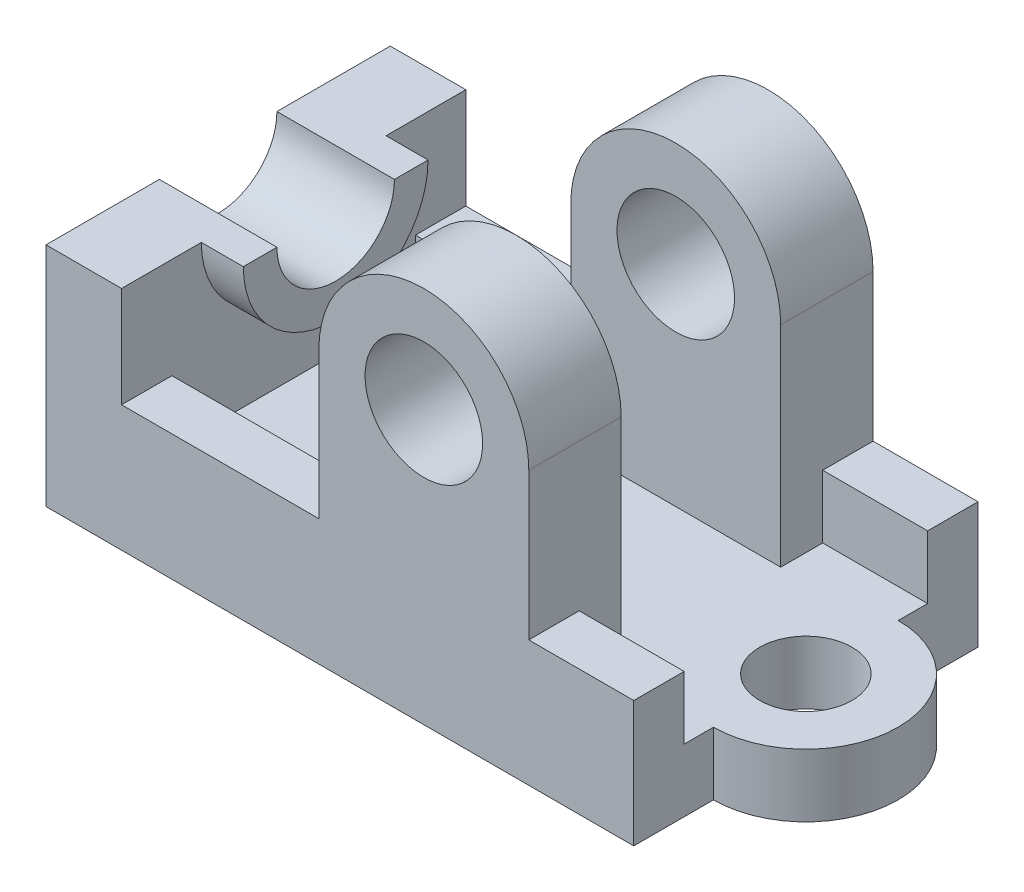
ISO-10303-21;
HEADER;
FILE_DESCRIPTION(('STEP AP214'),'2;1');
FILE_NAME('part.step','',(''),(''),'','','');
FILE_SCHEMA(('AUTOMOTIVE_DESIGN { 1 0 10303 214 1 1 1 1 }'));
ENDSEC;
DATA;
#1=APPLICATION_CONTEXT('core data for automotive mechanical design processes');
#2=APPLICATION_PROTOCOL_DEFINITION('international standard','automotive_design',2000,#1);
#3=PRODUCT_CONTEXT('',#1,'mechanical');
#4=PRODUCT('Part','Part','',(#3));
#5=PRODUCT_RELATED_PRODUCT_CATEGORY('part','',(#4));
#6=PRODUCT_DEFINITION_FORMATION('','',#4);
#7=PRODUCT_DEFINITION_CONTEXT('part definition',#1,'design');
#8=PRODUCT_DEFINITION('design','',#6,#7);
#9=PRODUCT_DEFINITION_SHAPE('','',#8);
#10=(LENGTH_UNIT() NAMED_UNIT(*) SI_UNIT(.MILLI.,.METRE.));
#11=(NAMED_UNIT(*) PLANE_ANGLE_UNIT() SI_UNIT($,.RADIAN.));
#12=(NAMED_UNIT(*) SI_UNIT($,.STERADIAN.) SOLID_ANGLE_UNIT());
#13=UNCERTAINTY_MEASURE_WITH_UNIT(LENGTH_MEASURE(1.E-05),#10,'distance_accuracy_value','');
#14=(GEOMETRIC_REPRESENTATION_CONTEXT(3) GLOBAL_UNCERTAINTY_ASSIGNED_CONTEXT((#13)) GLOBAL_UNIT_ASSIGNED_CONTEXT((#10,
#11,#12)) REPRESENTATION_CONTEXT('',''));
#15=CARTESIAN_POINT('',(0.,0.,0.));
#16=DIRECTION('',(0.,0.,1.));
#17=DIRECTION('',(1.,0.,0.));
#18=AXIS2_PLACEMENT_3D('',#15,#16,#17);
#19=CARTESIAN_POINT('',(140.,30.,41.));
#20=DIRECTION('',(-1.,0.,0.));
#21=DIRECTION('',(0.,0.,1.));
#22=AXIS2_PLACEMENT_3D('',#19,#20,#21);
#23=PLANE('',#22);
#24=DIRECTION('',(0.,0.,-1.));
#25=VECTOR('',#24,1.);
#26=CARTESIAN_POINT('',(140.,15.,41.));
#27=LINE('',#26,#25);
#28=CARTESIAN_POINT('',(140.,15.,-22.));
#29=VERTEX_POINT('',#28);
#30=CARTESIAN_POINT('',(140.,15.,-29.));
#31=VERTEX_POINT('',#30);
#32=EDGE_CURVE('E247',#29,#31,#27,.T.);
#33=ORIENTED_EDGE('',*,*,#32,.F.);
#34=DIRECTION('',(0.,-1.,0.));
#35=VECTOR('',#34,1.);
#36=CARTESIAN_POINT('',(140.,15.,-22.));
#37=LINE('',#36,#35);
#38=CARTESIAN_POINT('',(140.,0.,-22.));
#39=VERTEX_POINT('',#38);
#40=EDGE_CURVE('E229',#29,#39,#37,.T.);
#41=ORIENTED_EDGE('',*,*,#40,.T.);
#42=DIRECTION('',(0.,0.,-1.));
#43=VECTOR('',#42,1.);
#44=CARTESIAN_POINT('',(140.,0.,41.));
#45=LINE('',#44,#43);
#46=CARTESIAN_POINT('',(140.,0.,-41.));
#47=VERTEX_POINT('',#46);
#48=EDGE_CURVE('E293',#39,#47,#45,.T.);
#49=ORIENTED_EDGE('',*,*,#48,.T.);
#50=DIRECTION('',(0.,1.,0.));
#51=VECTOR('',#50,1.);
#52=CARTESIAN_POINT('',(140.,30.,-41.));
#53=LINE('',#52,#51);
#54=CARTESIAN_POINT('',(140.,30.,-41.));
#55=VERTEX_POINT('',#54);
#56=EDGE_CURVE('E272',#47,#55,#53,.T.);
#57=ORIENTED_EDGE('',*,*,#56,.T.);
#58=DIRECTION('',(0.,0.,-1.));
#59=VECTOR('',#58,1.);
#60=CARTESIAN_POINT('',(140.,30.,-29.));
#61=LINE('',#60,#59);
#62=CARTESIAN_POINT('',(140.,30.,-29.));
#63=VERTEX_POINT('',#62);
#64=EDGE_CURVE('E331',#63,#55,#61,.T.);
#65=ORIENTED_EDGE('',*,*,#64,.F.);
#66=DIRECTION('',(0.,-1.,0.));
#67=VECTOR('',#66,1.);
#68=CARTESIAN_POINT('',(140.,15.,-29.));
#69=LINE('',#68,#67);
#70=EDGE_CURVE('E325',#63,#31,#69,.T.);
#71=ORIENTED_EDGE('',*,*,#70,.T.);
#72=EDGE_LOOP('',(#33,#41,#49,#57,#65,#71));
#73=FACE_BOUND('',#72,.T.);
#74=ADVANCED_FACE('F41',(#73),#23,.F.);
#75=CARTESIAN_POINT('',(0.,54.,41.));
#76=DIRECTION('',(0.,-1.,0.));
#77=DIRECTION('',(0.,0.,-1.));
#78=AXIS2_PLACEMENT_3D('',#75,#76,#77);
#79=PLANE('',#78);
#80=DIRECTION('',(0.,0.,-1.));
#81=VECTOR('',#80,1.);
#82=CARTESIAN_POINT('',(0.,54.,41.));
#83=LINE('',#82,#81);
#84=CARTESIAN_POINT('',(0.,54.,-14.));
#85=VERTEX_POINT('',#84);
#86=CARTESIAN_POINT('',(0.,54.,-41.));
#87=VERTEX_POINT('',#86);
#88=EDGE_CURVE('E283',#85,#87,#83,.T.);
#89=ORIENTED_EDGE('',*,*,#88,.F.);
#90=DIRECTION('',(1.,0.,0.));
#91=VECTOR('',#90,1.);
#92=CARTESIAN_POINT('',(18.,54.,-14.));
#93=LINE('',#92,#91);
#94=CARTESIAN_POINT('',(28.,54.,-14.));
#95=VERTEX_POINT('',#94);
#96=EDGE_CURVE('E61',#85,#95,#93,.T.);
#97=ORIENTED_EDGE('',*,*,#96,.T.);
#98=DIRECTION('',(0.,0.,-1.));
#99=VECTOR('',#98,1.);
#100=CARTESIAN_POINT('',(28.,54.,0.));
#101=LINE('',#100,#99);
#102=CARTESIAN_POINT('',(28.,54.,-22.));
#103=VERTEX_POINT('',#102);
#104=EDGE_CURVE('E537',#95,#103,#101,.T.);
#105=ORIENTED_EDGE('',*,*,#104,.T.);
#106=DIRECTION('',(1.,0.,0.));
#107=VECTOR('',#106,1.);
#108=CARTESIAN_POINT('',(18.,54.,-22.));
#109=LINE('',#108,#107);
#110=CARTESIAN_POINT('',(18.,54.,-22.));
#111=VERTEX_POINT('',#110);
#112=EDGE_CURVE('E490',#111,#103,#109,.T.);
#113=ORIENTED_EDGE('',*,*,#112,.F.);
#114=DIRECTION('',(0.,0.,-1.));
#115=VECTOR('',#114,1.);
#116=CARTESIAN_POINT('',(18.,54.,41.));
#117=LINE('',#116,#115);
#118=CARTESIAN_POINT('',(18.,54.,-41.));
#119=VERTEX_POINT('',#118);
#120=EDGE_CURVE('E289',#111,#119,#117,.T.);
#121=ORIENTED_EDGE('',*,*,#120,.T.);
#122=DIRECTION('',(-1.,0.,0.));
#123=VECTOR('',#122,1.);
#124=CARTESIAN_POINT('',(0.,54.,-41.));
#125=LINE('',#124,#123);
#126=EDGE_CURVE('E280',#119,#87,#125,.T.);
#127=ORIENTED_EDGE('',*,*,#126,.T.);
#128=EDGE_LOOP('',(#89,#97,#105,#113,#121,#127));
#129=FACE_BOUND('',#128,.T.);
#130=ADVANCED_FACE('F446',(#129),#79,.F.);
#131=CARTESIAN_POINT('',(140.,30.,-29.));
#132=DIRECTION('',(0.,1.,0.));
#133=DIRECTION('',(0.,0.,1.));
#134=AXIS2_PLACEMENT_3D('',#131,#132,#133);
#135=PLANE('',#134);
#136=DIRECTION('',(0.,0.,1.));
#137=VECTOR('',#136,1.);
#138=CARTESIAN_POINT('',(65.,30.,-29.));
#139=LINE('',#138,#137);
#140=CARTESIAN_POINT('',(65.,30.,-41.));
#141=VERTEX_POINT('',#140);
#142=CARTESIAN_POINT('',(65.,30.,-29.));
#143=VERTEX_POINT('',#142);
#144=EDGE_CURVE('E406',#141,#143,#139,.T.);
#145=ORIENTED_EDGE('',*,*,#144,.F.);
#146=DIRECTION('',(1.,0.,0.));
#147=VECTOR('',#146,1.);
#148=CARTESIAN_POINT('',(140.,30.,-41.));
#149=LINE('',#148,#147);
#150=CARTESIAN_POINT('',(18.,30.,-41.));
#151=VERTEX_POINT('',#150);
#152=EDGE_CURVE('E329',#151,#141,#149,.T.);
#153=ORIENTED_EDGE('',*,*,#152,.F.);
#154=DIRECTION('',(0.,0.,-1.));
#155=VECTOR('',#154,1.);
#156=CARTESIAN_POINT('',(18.,30.,-29.));
#157=LINE('',#156,#155);
#158=CARTESIAN_POINT('',(18.,30.,-29.));
#159=VERTEX_POINT('',#158);
#160=EDGE_CURVE('E327',#159,#151,#157,.T.);
#161=ORIENTED_EDGE('',*,*,#160,.F.);
#162=DIRECTION('',(1.,0.,0.));
#163=VECTOR('',#162,1.);
#164=CARTESIAN_POINT('',(140.,30.,-29.));
#165=LINE('',#164,#163);
#166=EDGE_CURVE('E326',#159,#143,#165,.T.);
#167=ORIENTED_EDGE('',*,*,#166,.T.);
#168=EDGE_LOOP('',(#145,#153,#161,#167));
#169=FACE_BOUND('',#168,.T.);
#170=ADVANCED_FACE('F453',(#169),#135,.T.);
#171=CARTESIAN_POINT('',(0.,0.,-29.));
#172=DIRECTION('',(0.,0.,1.));
#173=DIRECTION('',(1.,0.,0.));
#174=AXIS2_PLACEMENT_3D('',#171,#172,#173);
#175=PLANE('',#174);
#176=DIRECTION('',(0.,-1.,0.));
#177=VECTOR('',#176,1.);
#178=CARTESIAN_POINT('',(65.,0.,-29.));
#179=LINE('',#178,#177);
#180=CARTESIAN_POINT('',(65.,15.,-29.));
#181=VERTEX_POINT('',#180);
#182=EDGE_CURVE('E11',#143,#181,#179,.T.);
#183=ORIENTED_EDGE('',*,*,#182,.F.);
#184=ORIENTED_EDGE('',*,*,#166,.F.);
#185=DIRECTION('',(0.,1.,0.));
#186=VECTOR('',#185,1.);
#187=CARTESIAN_POINT('',(18.,15.,-29.));
#188=LINE('',#187,#186);
#189=CARTESIAN_POINT('',(18.,15.,-29.));
#190=VERTEX_POINT('',#189);
#191=EDGE_CURVE('E320',#190,#159,#188,.T.);
#192=ORIENTED_EDGE('',*,*,#191,.F.);
#193=DIRECTION('',(-1.,0.,0.));
#194=VECTOR('',#193,1.);
#195=CARTESIAN_POINT('',(140.,15.,-29.));
#196=LINE('',#195,#194);
#197=EDGE_CURVE('E319',#181,#190,#196,.T.);
#198=ORIENTED_EDGE('',*,*,#197,.F.);
#199=EDGE_LOOP('',(#183,#184,#192,#198));
#200=FACE_BOUND('',#199,.T.);
#201=ADVANCED_FACE('F604',(#200),#175,.T.);
#202=CARTESIAN_POINT('',(18.,30.,29.));
#203=DIRECTION('',(0.,1.,0.));
#204=DIRECTION('',(0.,0.,1.));
#205=AXIS2_PLACEMENT_3D('',#202,#203,#204);
#206=PLANE('',#205);
#207=DIRECTION('',(0.,0.,1.));
#208=VECTOR('',#207,1.);
#209=CARTESIAN_POINT('',(65.,30.,29.));
#210=LINE('',#209,#208);
#211=CARTESIAN_POINT('',(65.,30.,29.));
#212=VERTEX_POINT('',#211);
#213=CARTESIAN_POINT('',(65.,30.,41.));
#214=VERTEX_POINT('',#213);
#215=EDGE_CURVE('E392',#212,#214,#210,.T.);
#216=ORIENTED_EDGE('',*,*,#215,.F.);
#217=DIRECTION('',(-1.,0.,0.));
#218=VECTOR('',#217,1.);
#219=CARTESIAN_POINT('',(18.,30.,29.));
#220=LINE('',#219,#218);
#221=CARTESIAN_POINT('',(18.,30.,29.));
#222=VERTEX_POINT('',#221);
#223=EDGE_CURVE('E348',#212,#222,#220,.T.);
#224=ORIENTED_EDGE('',*,*,#223,.T.);
#225=DIRECTION('',(0.,0.,1.));
#226=VECTOR('',#225,1.);
#227=CARTESIAN_POINT('',(18.,30.,29.));
#228=LINE('',#227,#226);
#229=CARTESIAN_POINT('',(18.,30.,41.));
#230=VERTEX_POINT('',#229);
#231=EDGE_CURVE('E254',#222,#230,#228,.T.);
#232=ORIENTED_EDGE('',*,*,#231,.T.);
#233=DIRECTION('',(-1.,0.,0.));
#234=VECTOR('',#233,1.);
#235=CARTESIAN_POINT('',(18.,30.,41.));
#236=LINE('',#235,#234);
#237=EDGE_CURVE('E340',#214,#230,#236,.T.);
#238=ORIENTED_EDGE('',*,*,#237,.F.);
#239=EDGE_LOOP('',(#216,#224,#232,#238));
#240=FACE_BOUND('',#239,.T.);
#241=ADVANCED_FACE('F472',(#240),#206,.T.);
#242=CARTESIAN_POINT('',(0.,0.,29.));
#243=DIRECTION('',(0.,0.,-1.));
#244=DIRECTION('',(-1.,0.,0.));
#245=AXIS2_PLACEMENT_3D('',#242,#243,#244);
#246=PLANE('',#245);
#247=DIRECTION('',(0.,1.,0.));
#248=VECTOR('',#247,1.);
#249=CARTESIAN_POINT('',(65.,0.,29.));
#250=LINE('',#249,#248);
#251=CARTESIAN_POINT('',(65.,15.,29.));
#252=VERTEX_POINT('',#251);
#253=EDGE_CURVE('E298',#252,#212,#250,.T.);
#254=ORIENTED_EDGE('',*,*,#253,.F.);
#255=DIRECTION('',(1.,0.,0.));
#256=VECTOR('',#255,1.);
#257=CARTESIAN_POINT('',(18.,15.,29.));
#258=LINE('',#257,#256);
#259=CARTESIAN_POINT('',(18.,15.,29.));
#260=VERTEX_POINT('',#259);
#261=EDGE_CURVE('E344',#260,#252,#258,.T.);
#262=ORIENTED_EDGE('',*,*,#261,.F.);
#263=DIRECTION('',(0.,-1.,0.));
#264=VECTOR('',#263,1.);
#265=CARTESIAN_POINT('',(18.,15.,29.));
#266=LINE('',#265,#264);
#267=EDGE_CURVE('E338',#222,#260,#266,.T.);
#268=ORIENTED_EDGE('',*,*,#267,.F.);
#269=ORIENTED_EDGE('',*,*,#223,.F.);
#270=EDGE_LOOP('',(#254,#262,#268,#269));
#271=FACE_BOUND('',#270,.T.);
#272=ADVANCED_FACE('F467',(#271),#246,.T.);
#273=CARTESIAN_POINT('',(140.,0.,41.));
#274=DIRECTION('',(0.,1.,0.));
#275=DIRECTION('',(0.,0.,1.));
#276=AXIS2_PLACEMENT_3D('',#273,#274,#275);
#277=PLANE('',#276);
#278=CARTESIAN_POINT('',(140.,0.,0.));
#279=DIRECTION('',(0.,-1.,0.));
#280=DIRECTION('',(0.,0.,-1.));
#281=AXIS2_PLACEMENT_3D('',#278,#279,#280);
#282=CIRCLE('',#281,11.);
#283=CARTESIAN_POINT('',(140.,0.,-11.));
#284=VERTEX_POINT('',#283);
#285=EDGE_CURVE('E478',#284,#284,#282,.T.);
#286=ORIENTED_EDGE('',*,*,#285,.F.);
#287=EDGE_LOOP('',(#286));
#288=FACE_BOUND('',#287,.T.);
#289=DIRECTION('',(1.,0.,0.));
#290=VECTOR('',#289,1.);
#291=CARTESIAN_POINT('',(140.,0.,-41.));
#292=LINE('',#291,#290);
#293=CARTESIAN_POINT('',(0.,0.,-41.));
#294=VERTEX_POINT('',#293);
#295=EDGE_CURVE('E252',#294,#47,#292,.T.);
#296=ORIENTED_EDGE('',*,*,#295,.T.);
#297=ORIENTED_EDGE('',*,*,#48,.F.);
#298=CARTESIAN_POINT('',(140.,0.,0.));
#299=DIRECTION('',(0.,-1.,0.));
#300=DIRECTION('',(0.,0.,-1.));
#301=AXIS2_PLACEMENT_3D('',#298,#299,#300);
#302=CIRCLE('',#301,22.);
#303=CARTESIAN_POINT('',(140.,0.,22.));
#304=VERTEX_POINT('',#303);
#305=EDGE_CURVE('E235',#39,#304,#302,.T.);
#306=ORIENTED_EDGE('',*,*,#305,.T.);
#307=CARTESIAN_POINT('',(140.,0.,41.));
#308=VERTEX_POINT('',#307);
#309=EDGE_CURVE('E245',#308,#304,#45,.T.);
#310=ORIENTED_EDGE('',*,*,#309,.F.);
#311=DIRECTION('',(1.,0.,0.));
#312=VECTOR('',#311,1.);
#313=CARTESIAN_POINT('',(140.,0.,41.));
#314=LINE('',#313,#312);
#315=CARTESIAN_POINT('',(0.,0.,41.));
#316=VERTEX_POINT('',#315);
#317=EDGE_CURVE('E257',#316,#308,#314,.T.);
#318=ORIENTED_EDGE('',*,*,#317,.F.);
#319=DIRECTION('',(0.,0.,-1.));
#320=VECTOR('',#319,1.);
#321=CARTESIAN_POINT('',(0.,0.,41.));
#322=LINE('',#321,#320);
#323=EDGE_CURVE('E270',#316,#294,#322,.T.);
#324=ORIENTED_EDGE('',*,*,#323,.T.);
#325=EDGE_LOOP('',(#296,#297,#306,#310,#318,#324));
#326=FACE_BOUND('',#325,.T.);
#327=ADVANCED_FACE('F43',(#288,#326),#277,.F.);
#328=ORIENTED_EDGE('',*,*,#309,.T.);
#329=DIRECTION('',(0.,-1.,0.));
#330=VECTOR('',#329,1.);
#331=CARTESIAN_POINT('',(140.,15.,22.));
#332=LINE('',#331,#330);
#333=CARTESIAN_POINT('',(140.,15.,22.));
#334=VERTEX_POINT('',#333);
#335=EDGE_CURVE('E227',#334,#304,#332,.T.);
#336=ORIENTED_EDGE('',*,*,#335,.F.);
#337=CARTESIAN_POINT('',(140.,15.,29.));
#338=VERTEX_POINT('',#337);
#339=EDGE_CURVE('E237',#338,#334,#27,.T.);
#340=ORIENTED_EDGE('',*,*,#339,.F.);
#341=DIRECTION('',(0.,1.,0.));
#342=VECTOR('',#341,1.);
#343=CARTESIAN_POINT('',(140.,15.,29.));
#344=LINE('',#343,#342);
#345=CARTESIAN_POINT('',(140.,30.,29.));
#346=VERTEX_POINT('',#345);
#347=EDGE_CURVE('E346',#338,#346,#344,.T.);
#348=ORIENTED_EDGE('',*,*,#347,.T.);
#349=DIRECTION('',(0.,0.,1.));
#350=VECTOR('',#349,1.);
#351=CARTESIAN_POINT('',(140.,30.,29.));
#352=LINE('',#351,#350);
#353=CARTESIAN_POINT('',(140.,30.,41.));
#354=VERTEX_POINT('',#353);
#355=EDGE_CURVE('E354',#346,#354,#352,.T.);
#356=ORIENTED_EDGE('',*,*,#355,.T.);
#357=DIRECTION('',(0.,1.,0.));
#358=VECTOR('',#357,1.);
#359=CARTESIAN_POINT('',(140.,30.,41.));
#360=LINE('',#359,#358);
#361=EDGE_CURVE('E256',#308,#354,#360,.T.);
#362=ORIENTED_EDGE('',*,*,#361,.F.);
#363=EDGE_LOOP('',(#328,#336,#340,#348,#356,#362));
#364=FACE_BOUND('',#363,.T.);
#365=ADVANCED_FACE('F240',(#364),#23,.F.);
#366=CARTESIAN_POINT('',(18.,54.,41.));
#367=DIRECTION('',(-1.,0.,0.));
#368=DIRECTION('',(0.,-1.,0.));
#369=AXIS2_PLACEMENT_3D('',#366,#367,#368);
#370=PLANE('',#369);
#371=CARTESIAN_POINT('',(18.,54.,0.));
#372=DIRECTION('',(1.,0.,0.));
#373=DIRECTION('',(0.,1.,0.));
#374=AXIS2_PLACEMENT_3D('',#371,#372,#373);
#375=CIRCLE('',#374,22.);
#376=CARTESIAN_POINT('',(18.,54.,22.));
#377=VERTEX_POINT('',#376);
#378=EDGE_CURVE('E529',#377,#111,#375,.T.);
#379=ORIENTED_EDGE('',*,*,#378,.F.);
#380=CARTESIAN_POINT('',(18.,54.,41.));
#381=VERTEX_POINT('',#380);
#382=EDGE_CURVE('E290',#381,#377,#117,.T.);
#383=ORIENTED_EDGE('',*,*,#382,.F.);
#384=DIRECTION('',(0.,1.,0.));
#385=VECTOR('',#384,1.);
#386=CARTESIAN_POINT('',(18.,54.,41.));
#387=LINE('',#386,#385);
#388=EDGE_CURVE('E265',#230,#381,#387,.T.);
#389=ORIENTED_EDGE('',*,*,#388,.F.);
#390=ORIENTED_EDGE('',*,*,#231,.F.);
#391=ORIENTED_EDGE('',*,*,#267,.T.);
#392=DIRECTION('',(0.,0.,-1.));
#393=VECTOR('',#392,1.);
#394=CARTESIAN_POINT('',(18.,15.,41.));
#395=LINE('',#394,#393);
#396=EDGE_CURVE('E250',#260,#190,#395,.T.);
#397=ORIENTED_EDGE('',*,*,#396,.T.);
#398=ORIENTED_EDGE('',*,*,#191,.T.);
#399=ORIENTED_EDGE('',*,*,#160,.T.);
#400=DIRECTION('',(0.,1.,0.));
#401=VECTOR('',#400,1.);
#402=CARTESIAN_POINT('',(18.,54.,-41.));
#403=LINE('',#402,#401);
#404=EDGE_CURVE('E274',#151,#119,#403,.T.);
#405=ORIENTED_EDGE('',*,*,#404,.T.);
#406=ORIENTED_EDGE('',*,*,#120,.F.);
#407=EDGE_LOOP('',(#379,#383,#389,#390,#391,#397,#398,#399,#405,#406));
#408=FACE_BOUND('',#407,.T.);
#409=ADVANCED_FACE('F457',(#408),#370,.F.);
#410=DIRECTION('',(1.,0.,0.));
#411=VECTOR('',#410,1.);
#412=CARTESIAN_POINT('',(18.,54.,14.));
#413=LINE('',#412,#411);
#414=CARTESIAN_POINT('',(0.,54.,14.));
#415=VERTEX_POINT('',#414);
#416=CARTESIAN_POINT('',(28.,54.,14.));
#417=VERTEX_POINT('',#416);
#418=EDGE_CURVE('E533',#415,#417,#413,.T.);
#419=ORIENTED_EDGE('',*,*,#418,.F.);
#420=CARTESIAN_POINT('',(0.,54.,41.));
#421=VERTEX_POINT('',#420);
#422=EDGE_CURVE('E282',#421,#415,#83,.T.);
#423=ORIENTED_EDGE('',*,*,#422,.F.);
#424=DIRECTION('',(-1.,0.,0.));
#425=VECTOR('',#424,1.);
#426=CARTESIAN_POINT('',(0.,54.,41.));
#427=LINE('',#426,#425);
#428=EDGE_CURVE('E262',#381,#421,#427,.T.);
#429=ORIENTED_EDGE('',*,*,#428,.F.);
#430=ORIENTED_EDGE('',*,*,#382,.T.);
#431=DIRECTION('',(1.,0.,0.));
#432=VECTOR('',#431,1.);
#433=CARTESIAN_POINT('',(18.,54.,22.));
#434=LINE('',#433,#432);
#435=CARTESIAN_POINT('',(28.,54.,22.));
#436=VERTEX_POINT('',#435);
#437=EDGE_CURVE('E531',#377,#436,#434,.T.);
#438=ORIENTED_EDGE('',*,*,#437,.T.);
#439=EDGE_CURVE('E541',#436,#417,#101,.T.);
#440=ORIENTED_EDGE('',*,*,#439,.T.);
#441=EDGE_LOOP('',(#419,#423,#429,#430,#438,#440));
#442=FACE_BOUND('',#441,.T.);
#443=ADVANCED_FACE('F443',(#442),#79,.F.);
#444=CARTESIAN_POINT('',(0.,0.,41.));
#445=DIRECTION('',(1.,0.,0.));
#446=DIRECTION('',(0.,0.,-1.));
#447=AXIS2_PLACEMENT_3D('',#444,#445,#446);
#448=PLANE('',#447);
#449=ORIENTED_EDGE('',*,*,#422,.T.);
#450=CARTESIAN_POINT('',(0.,54.,0.));
#451=DIRECTION('',(1.,0.,0.));
#452=DIRECTION('',(0.,1.,0.));
#453=AXIS2_PLACEMENT_3D('',#450,#451,#452);
#454=CIRCLE('',#453,14.);
#455=EDGE_CURVE('E488',#415,#85,#454,.T.);
#456=ORIENTED_EDGE('',*,*,#455,.T.);
#457=ORIENTED_EDGE('',*,*,#88,.T.);
#458=DIRECTION('',(0.,-1.,0.));
#459=VECTOR('',#458,1.);
#460=CARTESIAN_POINT('',(0.,0.,-41.));
#461=LINE('',#460,#459);
#462=EDGE_CURVE('E258',#87,#294,#461,.T.);
#463=ORIENTED_EDGE('',*,*,#462,.T.);
#464=ORIENTED_EDGE('',*,*,#323,.F.);
#465=DIRECTION('',(0.,-1.,0.));
#466=VECTOR('',#465,1.);
#467=CARTESIAN_POINT('',(0.,0.,41.));
#468=LINE('',#467,#466);
#469=EDGE_CURVE('E267',#421,#316,#468,.T.);
#470=ORIENTED_EDGE('',*,*,#469,.F.);
#471=EDGE_LOOP('',(#449,#456,#457,#463,#464,#470));
#472=FACE_BOUND('',#471,.T.);
#473=ADVANCED_FACE('F432',(#472),#448,.F.);
#474=CARTESIAN_POINT('',(0.,0.,41.));
#475=DIRECTION('',(0.,0.,-1.));
#476=DIRECTION('',(-1.,0.,0.));
#477=AXIS2_PLACEMENT_3D('',#474,#475,#476);
#478=PLANE('',#477);
#479=DIRECTION('',(0.,-1.,0.));
#480=VECTOR('',#479,1.);
#481=CARTESIAN_POINT('',(65.,0.,41.));
#482=LINE('',#481,#480);
#483=CARTESIAN_POINT('',(65.,65.,41.));
#484=VERTEX_POINT('',#483);
#485=EDGE_CURVE('E380',#484,#214,#482,.T.);
#486=ORIENTED_EDGE('',*,*,#485,.T.);
#487=ORIENTED_EDGE('',*,*,#237,.T.);
#488=ORIENTED_EDGE('',*,*,#388,.T.);
#489=ORIENTED_EDGE('',*,*,#428,.T.);
#490=ORIENTED_EDGE('',*,*,#469,.T.);
#491=ORIENTED_EDGE('',*,*,#317,.T.);
#492=ORIENTED_EDGE('',*,*,#361,.T.);
#493=CARTESIAN_POINT('',(115.,30.,41.));
#494=VERTEX_POINT('',#493);
#495=EDGE_CURVE('E345',#354,#494,#236,.T.);
#496=ORIENTED_EDGE('',*,*,#495,.T.);
#497=DIRECTION('',(0.,1.,0.));
#498=VECTOR('',#497,1.);
#499=CARTESIAN_POINT('',(115.,0.,41.));
#500=LINE('',#499,#498);
#501=CARTESIAN_POINT('',(115.,65.,41.));
#502=VERTEX_POINT('',#501);
#503=EDGE_CURVE('E367',#494,#502,#500,.T.);
#504=ORIENTED_EDGE('',*,*,#503,.T.);
#505=CARTESIAN_POINT('',(90.,65.,41.));
#506=DIRECTION('',(0.,0.,1.));
#507=DIRECTION('',(1.,0.,0.));
#508=AXIS2_PLACEMENT_3D('',#505,#506,#507);
#509=CIRCLE('',#508,25.);
#510=EDGE_CURVE('E376',#502,#484,#509,.T.);
#511=ORIENTED_EDGE('',*,*,#510,.T.);
#512=EDGE_LOOP('',(#486,#487,#488,#489,#490,#491,#492,#496,#504,#511));
#513=FACE_BOUND('',#512,.T.);
#514=CARTESIAN_POINT('',(90.,65.,41.));
#515=DIRECTION('',(0.,0.,1.));
#516=DIRECTION('',(1.,0.,0.));
#517=AXIS2_PLACEMENT_3D('',#514,#515,#516);
#518=CIRCLE('',#517,14.);
#519=CARTESIAN_POINT('',(104.,65.,41.));
#520=VERTEX_POINT('',#519);
#521=EDGE_CURVE('E382',#520,#520,#518,.T.);
#522=ORIENTED_EDGE('',*,*,#521,.F.);
#523=EDGE_LOOP('',(#522));
#524=FACE_BOUND('',#523,.T.);
#525=ADVANCED_FACE('F366',(#513,#524),#478,.F.);
#526=CARTESIAN_POINT('',(0.,0.,-41.));
#527=DIRECTION('',(0.,0.,-1.));
#528=DIRECTION('',(-1.,0.,0.));
#529=AXIS2_PLACEMENT_3D('',#526,#527,#528);
#530=PLANE('',#529);
#531=CARTESIAN_POINT('',(90.,64.9999999999999,-41.));
#532=DIRECTION('',(0.,0.,-1.));
#533=DIRECTION('',(-1.,0.,0.));
#534=AXIS2_PLACEMENT_3D('',#531,#532,#533);
#535=CIRCLE('',#534,14.);
#536=CARTESIAN_POINT('',(76.,64.9999999999999,-41.));
#537=VERTEX_POINT('',#536);
#538=EDGE_CURVE('E504',#537,#537,#535,.T.);
#539=ORIENTED_EDGE('',*,*,#538,.F.);
#540=EDGE_LOOP('',(#539));
#541=FACE_BOUND('',#540,.T.);
#542=ORIENTED_EDGE('',*,*,#152,.T.);
#543=DIRECTION('',(0.,1.,0.));
#544=VECTOR('',#543,1.);
#545=CARTESIAN_POINT('',(65.,0.,-41.));
#546=LINE('',#545,#544);
#547=CARTESIAN_POINT('',(65.,65.,-41.));
#548=VERTEX_POINT('',#547);
#549=EDGE_CURVE('E491',#141,#548,#546,.T.);
#550=ORIENTED_EDGE('',*,*,#549,.T.);
#551=CARTESIAN_POINT('',(90.,65.,-41.));
#552=DIRECTION('',(0.,0.,-1.));
#553=DIRECTION('',(-1.,0.,0.));
#554=AXIS2_PLACEMENT_3D('',#551,#552,#553);
#555=CIRCLE('',#554,25.);
#556=CARTESIAN_POINT('',(115.,65.,-41.));
#557=VERTEX_POINT('',#556);
#558=EDGE_CURVE('E499',#548,#557,#555,.T.);
#559=ORIENTED_EDGE('',*,*,#558,.T.);
#560=DIRECTION('',(0.,-1.,0.));
#561=VECTOR('',#560,1.);
#562=CARTESIAN_POINT('',(115.,0.,-41.));
#563=LINE('',#562,#561);
#564=CARTESIAN_POINT('',(115.,30.,-41.));
#565=VERTEX_POINT('',#564);
#566=EDGE_CURVE('E401',#557,#565,#563,.T.);
#567=ORIENTED_EDGE('',*,*,#566,.T.);
#568=EDGE_CURVE('E335',#565,#55,#149,.T.);
#569=ORIENTED_EDGE('',*,*,#568,.T.);
#570=ORIENTED_EDGE('',*,*,#56,.F.);
#571=ORIENTED_EDGE('',*,*,#295,.F.);
#572=ORIENTED_EDGE('',*,*,#462,.F.);
#573=ORIENTED_EDGE('',*,*,#126,.F.);
#574=ORIENTED_EDGE('',*,*,#404,.F.);
#575=EDGE_LOOP('',(#542,#550,#559,#567,#569,#570,#571,#572,#573,#574));
#576=FACE_BOUND('',#575,.T.);
#577=ADVANCED_FACE('F398',(#541,#576),#530,.T.);
#578=CARTESIAN_POINT('',(18.,15.,41.));
#579=DIRECTION('',(0.,-1.,0.));
#580=DIRECTION('',(0.,0.,-1.));
#581=AXIS2_PLACEMENT_3D('',#578,#579,#580);
#582=PLANE('',#581);
#583=CARTESIAN_POINT('',(140.,15.,0.));
#584=DIRECTION('',(0.,-1.,0.));
#585=DIRECTION('',(0.,0.,-1.));
#586=AXIS2_PLACEMENT_3D('',#583,#584,#585);
#587=CIRCLE('',#586,11.);
#588=CARTESIAN_POINT('',(140.,15.,-11.));
#589=VERTEX_POINT('',#588);
#590=EDGE_CURVE('E544',#589,#589,#587,.T.);
#591=ORIENTED_EDGE('',*,*,#590,.T.);
#592=EDGE_LOOP('',(#591));
#593=FACE_BOUND('',#592,.T.);
#594=DIRECTION('',(-1.,0.,0.));
#595=VECTOR('',#594,1.);
#596=CARTESIAN_POINT('',(0.,15.,-19.));
#597=LINE('',#596,#595);
#598=CARTESIAN_POINT('',(115.,15.,-19.));
#599=VERTEX_POINT('',#598);
#600=CARTESIAN_POINT('',(65.,15.,-19.));
#601=VERTEX_POINT('',#600);
#602=EDGE_CURVE('E507',#599,#601,#597,.T.);
#603=ORIENTED_EDGE('',*,*,#602,.T.);
#604=DIRECTION('',(0.,0.,-1.));
#605=VECTOR('',#604,1.);
#606=CARTESIAN_POINT('',(65.,15.,-19.));
#607=LINE('',#606,#605);
#608=EDGE_CURVE('E408',#601,#181,#607,.T.);
#609=ORIENTED_EDGE('',*,*,#608,.T.);
#610=ORIENTED_EDGE('',*,*,#197,.T.);
#611=ORIENTED_EDGE('',*,*,#396,.F.);
#612=ORIENTED_EDGE('',*,*,#261,.T.);
#613=DIRECTION('',(0.,0.,1.));
#614=VECTOR('',#613,1.);
#615=CARTESIAN_POINT('',(65.,15.,19.));
#616=LINE('',#615,#614);
#617=CARTESIAN_POINT('',(65.,15.,19.));
#618=VERTEX_POINT('',#617);
#619=EDGE_CURVE('E388',#618,#252,#616,.T.);
#620=ORIENTED_EDGE('',*,*,#619,.F.);
#621=DIRECTION('',(1.,0.,0.));
#622=VECTOR('',#621,1.);
#623=CARTESIAN_POINT('',(0.,15.,19.));
#624=LINE('',#623,#622);
#625=CARTESIAN_POINT('',(115.,15.,19.));
#626=VERTEX_POINT('',#625);
#627=EDGE_CURVE('E425',#618,#626,#624,.T.);
#628=ORIENTED_EDGE('',*,*,#627,.T.);
#629=DIRECTION('',(0.,0.,1.));
#630=VECTOR('',#629,1.);
#631=CARTESIAN_POINT('',(115.,15.,19.));
#632=LINE('',#631,#630);
#633=CARTESIAN_POINT('',(115.,15.,29.));
#634=VERTEX_POINT('',#633);
#635=EDGE_CURVE('E389',#626,#634,#632,.T.);
#636=ORIENTED_EDGE('',*,*,#635,.T.);
#637=EDGE_CURVE('E246',#634,#338,#258,.T.);
#638=ORIENTED_EDGE('',*,*,#637,.T.);
#639=ORIENTED_EDGE('',*,*,#339,.T.);
#640=CARTESIAN_POINT('',(140.,15.,0.));
#641=DIRECTION('',(0.,-1.,0.));
#642=DIRECTION('',(0.,0.,-1.));
#643=AXIS2_PLACEMENT_3D('',#640,#641,#642);
#644=CIRCLE('',#643,22.);
#645=EDGE_CURVE('E57',#29,#334,#644,.T.);
#646=ORIENTED_EDGE('',*,*,#645,.F.);
#647=ORIENTED_EDGE('',*,*,#32,.T.);
#648=CARTESIAN_POINT('',(115.,15.,-29.));
#649=VERTEX_POINT('',#648);
#650=EDGE_CURVE('E313',#31,#649,#196,.T.);
#651=ORIENTED_EDGE('',*,*,#650,.T.);
#652=DIRECTION('',(0.,0.,-1.));
#653=VECTOR('',#652,1.);
#654=CARTESIAN_POINT('',(115.,15.,-19.));
#655=LINE('',#654,#653);
#656=EDGE_CURVE('E308',#599,#649,#655,.T.);
#657=ORIENTED_EDGE('',*,*,#656,.F.);
#658=EDGE_LOOP('',(#603,#609,#610,#611,#612,#620,#628,#636,#638,#639,#646,#647,#651,#657));
#659=FACE_BOUND('',#658,.T.);
#660=ADVANCED_FACE('F242',(#593,#659),#582,.F.);
#661=DIRECTION('',(0.,0.,-1.));
#662=VECTOR('',#661,1.);
#663=CARTESIAN_POINT('',(115.,30.,29.));
#664=LINE('',#663,#662);
#665=CARTESIAN_POINT('',(115.,30.,29.));
#666=VERTEX_POINT('',#665);
#667=EDGE_CURVE('E365',#494,#666,#664,.T.);
#668=ORIENTED_EDGE('',*,*,#667,.F.);
#669=ORIENTED_EDGE('',*,*,#495,.F.);
#670=ORIENTED_EDGE('',*,*,#355,.F.);
#671=EDGE_CURVE('E347',#346,#666,#220,.T.);
#672=ORIENTED_EDGE('',*,*,#671,.T.);
#673=EDGE_LOOP('',(#668,#669,#670,#672));
#674=FACE_BOUND('',#673,.T.);
#675=ADVANCED_FACE('F359',(#674),#206,.T.);
#676=DIRECTION('',(0.,-1.,0.));
#677=VECTOR('',#676,1.);
#678=CARTESIAN_POINT('',(115.,0.,29.));
#679=LINE('',#678,#677);
#680=EDGE_CURVE('E291',#666,#634,#679,.T.);
#681=ORIENTED_EDGE('',*,*,#680,.F.);
#682=ORIENTED_EDGE('',*,*,#671,.F.);
#683=ORIENTED_EDGE('',*,*,#347,.F.);
#684=ORIENTED_EDGE('',*,*,#637,.F.);
#685=EDGE_LOOP('',(#681,#682,#683,#684));
#686=FACE_BOUND('',#685,.T.);
#687=ADVANCED_FACE('F471',(#686),#246,.T.);
#688=DIRECTION('',(0.,0.,-1.));
#689=VECTOR('',#688,1.);
#690=CARTESIAN_POINT('',(115.,30.,-29.));
#691=LINE('',#690,#689);
#692=CARTESIAN_POINT('',(115.,30.,-29.));
#693=VERTEX_POINT('',#692);
#694=EDGE_CURVE('E304',#693,#565,#691,.T.);
#695=ORIENTED_EDGE('',*,*,#694,.F.);
#696=EDGE_CURVE('E317',#693,#63,#165,.T.);
#697=ORIENTED_EDGE('',*,*,#696,.T.);
#698=ORIENTED_EDGE('',*,*,#64,.T.);
#699=ORIENTED_EDGE('',*,*,#568,.F.);
#700=EDGE_LOOP('',(#695,#697,#698,#699));
#701=FACE_BOUND('',#700,.T.);
#702=ADVANCED_FACE('F409',(#701),#135,.T.);
#703=DIRECTION('',(0.,1.,0.));
#704=VECTOR('',#703,1.);
#705=CARTESIAN_POINT('',(115.,0.,-29.));
#706=LINE('',#705,#704);
#707=EDGE_CURVE('E47',#649,#693,#706,.T.);
#708=ORIENTED_EDGE('',*,*,#707,.F.);
#709=ORIENTED_EDGE('',*,*,#650,.F.);
#710=ORIENTED_EDGE('',*,*,#70,.F.);
#711=ORIENTED_EDGE('',*,*,#696,.F.);
#712=EDGE_LOOP('',(#708,#709,#710,#711));
#713=FACE_BOUND('',#712,.T.);
#714=ADVANCED_FACE('F315',(#713),#175,.T.);
#715=CARTESIAN_POINT('',(65.,0.,19.));
#716=DIRECTION('',(-1.,0.,0.));
#717=DIRECTION('',(0.,0.,1.));
#718=AXIS2_PLACEMENT_3D('',#715,#716,#717);
#719=PLANE('',#718);
#720=ORIENTED_EDGE('',*,*,#253,.T.);
#721=ORIENTED_EDGE('',*,*,#215,.T.);
#722=ORIENTED_EDGE('',*,*,#485,.F.);
#723=DIRECTION('',(0.,0.,1.));
#724=VECTOR('',#723,1.);
#725=CARTESIAN_POINT('',(65.,65.,19.));
#726=LINE('',#725,#724);
#727=CARTESIAN_POINT('',(65.,65.,19.));
#728=VERTEX_POINT('',#727);
#729=EDGE_CURVE('E383',#728,#484,#726,.T.);
#730=ORIENTED_EDGE('',*,*,#729,.F.);
#731=DIRECTION('',(0.,-1.,0.));
#732=VECTOR('',#731,1.);
#733=CARTESIAN_POINT('',(65.,0.,19.));
#734=LINE('',#733,#732);
#735=EDGE_CURVE('E423',#728,#618,#734,.T.);
#736=ORIENTED_EDGE('',*,*,#735,.T.);
#737=ORIENTED_EDGE('',*,*,#619,.T.);
#738=EDGE_LOOP('',(#720,#721,#722,#730,#736,#737));
#739=FACE_BOUND('',#738,.T.);
#740=ADVANCED_FACE('F594',(#739),#719,.T.);
#741=CARTESIAN_POINT('',(90.,65.,19.));
#742=DIRECTION('',(0.,0.,1.));
#743=DIRECTION('',(1.,0.,0.));
#744=AXIS2_PLACEMENT_3D('',#741,#742,#743);
#745=CYLINDRICAL_SURFACE('',#744,25.);
#746=ORIENTED_EDGE('',*,*,#510,.F.);
#747=DIRECTION('',(0.,0.,1.));
#748=VECTOR('',#747,1.);
#749=CARTESIAN_POINT('',(115.,65.,19.));
#750=LINE('',#749,#748);
#751=CARTESIAN_POINT('',(115.,65.,19.));
#752=VERTEX_POINT('',#751);
#753=EDGE_CURVE('E372',#752,#502,#750,.T.);
#754=ORIENTED_EDGE('',*,*,#753,.F.);
#755=CARTESIAN_POINT('',(90.,65.,19.));
#756=DIRECTION('',(0.,0.,1.));
#757=DIRECTION('',(1.,0.,0.));
#758=AXIS2_PLACEMENT_3D('',#755,#756,#757);
#759=CIRCLE('',#758,25.);
#760=EDGE_CURVE('E393',#752,#728,#759,.T.);
#761=ORIENTED_EDGE('',*,*,#760,.T.);
#762=ORIENTED_EDGE('',*,*,#729,.T.);
#763=EDGE_LOOP('',(#746,#754,#761,#762));
#764=FACE_BOUND('',#763,.T.);
#765=ADVANCED_FACE('F587',(#764),#745,.T.);
#766=CARTESIAN_POINT('',(115.,0.,19.));
#767=DIRECTION('',(1.,0.,0.));
#768=DIRECTION('',(0.,0.,-1.));
#769=AXIS2_PLACEMENT_3D('',#766,#767,#768);
#770=PLANE('',#769);
#771=ORIENTED_EDGE('',*,*,#503,.F.);
#772=ORIENTED_EDGE('',*,*,#667,.T.);
#773=ORIENTED_EDGE('',*,*,#680,.T.);
#774=ORIENTED_EDGE('',*,*,#635,.F.);
#775=DIRECTION('',(0.,1.,0.));
#776=VECTOR('',#775,1.);
#777=CARTESIAN_POINT('',(115.,0.,19.));
#778=LINE('',#777,#776);
#779=EDGE_CURVE('E428',#626,#752,#778,.T.);
#780=ORIENTED_EDGE('',*,*,#779,.T.);
#781=ORIENTED_EDGE('',*,*,#753,.T.);
#782=EDGE_LOOP('',(#771,#772,#773,#774,#780,#781));
#783=FACE_BOUND('',#782,.T.);
#784=ADVANCED_FACE('F375',(#783),#770,.T.);
#785=CARTESIAN_POINT('',(90.,65.,19.));
#786=DIRECTION('',(0.,0.,1.));
#787=DIRECTION('',(1.,0.,0.));
#788=AXIS2_PLACEMENT_3D('',#785,#786,#787);
#789=CYLINDRICAL_SURFACE('',#788,14.);
#790=CARTESIAN_POINT('',(90.,65.,19.));
#791=DIRECTION('',(0.,0.,1.));
#792=DIRECTION('',(1.,0.,0.));
#793=AXIS2_PLACEMENT_3D('',#790,#791,#792);
#794=CIRCLE('',#793,14.);
#795=CARTESIAN_POINT('',(104.,65.,19.));
#796=VERTEX_POINT('',#795);
#797=EDGE_CURVE('E378',#796,#796,#794,.T.);
#798=ORIENTED_EDGE('',*,*,#797,.F.);
#799=EDGE_LOOP('',(#798));
#800=FACE_BOUND('',#799,.T.);
#801=ORIENTED_EDGE('',*,*,#521,.T.);
#802=EDGE_LOOP('',(#801));
#803=FACE_BOUND('',#802,.T.);
#804=ADVANCED_FACE('F435',(#800,#803),#789,.F.);
#805=CARTESIAN_POINT('',(0.,0.,19.));
#806=DIRECTION('',(0.,0.,1.));
#807=DIRECTION('',(1.,0.,0.));
#808=AXIS2_PLACEMENT_3D('',#805,#806,#807);
#809=PLANE('',#808);
#810=ORIENTED_EDGE('',*,*,#797,.T.);
#811=EDGE_LOOP('',(#810));
#812=FACE_BOUND('',#811,.T.);
#813=ORIENTED_EDGE('',*,*,#735,.F.);
#814=ORIENTED_EDGE('',*,*,#760,.F.);
#815=ORIENTED_EDGE('',*,*,#779,.F.);
#816=ORIENTED_EDGE('',*,*,#627,.F.);
#817=EDGE_LOOP('',(#813,#814,#815,#816));
#818=FACE_BOUND('',#817,.T.);
#819=ADVANCED_FACE('F583',(#812,#818),#809,.F.);
#820=CARTESIAN_POINT('',(65.,0.,-19.));
#821=DIRECTION('',(-1.,0.,0.));
#822=DIRECTION('',(0.,0.,1.));
#823=AXIS2_PLACEMENT_3D('',#820,#821,#822);
#824=PLANE('',#823);
#825=ORIENTED_EDGE('',*,*,#549,.F.);
#826=ORIENTED_EDGE('',*,*,#144,.T.);
#827=ORIENTED_EDGE('',*,*,#182,.T.);
#828=ORIENTED_EDGE('',*,*,#608,.F.);
#829=DIRECTION('',(0.,1.,0.));
#830=VECTOR('',#829,1.);
#831=CARTESIAN_POINT('',(65.,0.,-19.));
#832=LINE('',#831,#830);
#833=CARTESIAN_POINT('',(65.,65.,-19.));
#834=VERTEX_POINT('',#833);
#835=EDGE_CURVE('E512',#601,#834,#832,.T.);
#836=ORIENTED_EDGE('',*,*,#835,.T.);
#837=DIRECTION('',(0.,0.,-1.));
#838=VECTOR('',#837,1.);
#839=CARTESIAN_POINT('',(65.,65.,-19.));
#840=LINE('',#839,#838);
#841=EDGE_CURVE('E417',#834,#548,#840,.T.);
#842=ORIENTED_EDGE('',*,*,#841,.T.);
#843=EDGE_LOOP('',(#825,#826,#827,#828,#836,#842));
#844=FACE_BOUND('',#843,.T.);
#845=ADVANCED_FACE('F500',(#844),#824,.T.);
#846=CARTESIAN_POINT('',(115.,0.,-19.));
#847=DIRECTION('',(1.,0.,0.));
#848=DIRECTION('',(0.,0.,-1.));
#849=AXIS2_PLACEMENT_3D('',#846,#847,#848);
#850=PLANE('',#849);
#851=ORIENTED_EDGE('',*,*,#707,.T.);
#852=ORIENTED_EDGE('',*,*,#694,.T.);
#853=ORIENTED_EDGE('',*,*,#566,.F.);
#854=DIRECTION('',(0.,0.,-1.));
#855=VECTOR('',#854,1.);
#856=CARTESIAN_POINT('',(115.,65.,-19.));
#857=LINE('',#856,#855);
#858=CARTESIAN_POINT('',(115.,65.,-19.));
#859=VERTEX_POINT('',#858);
#860=EDGE_CURVE('E514',#859,#557,#857,.T.);
#861=ORIENTED_EDGE('',*,*,#860,.F.);
#862=DIRECTION('',(0.,-1.,0.));
#863=VECTOR('',#862,1.);
#864=CARTESIAN_POINT('',(115.,0.,-19.));
#865=LINE('',#864,#863);
#866=EDGE_CURVE('E517',#859,#599,#865,.T.);
#867=ORIENTED_EDGE('',*,*,#866,.T.);
#868=ORIENTED_EDGE('',*,*,#656,.T.);
#869=EDGE_LOOP('',(#851,#852,#853,#861,#867,#868));
#870=FACE_BOUND('',#869,.T.);
#871=ADVANCED_FACE('F305',(#870),#850,.T.);
#872=CARTESIAN_POINT('',(90.,65.,-19.));
#873=DIRECTION('',(0.,0.,-1.));
#874=DIRECTION('',(-1.,0.,0.));
#875=AXIS2_PLACEMENT_3D('',#872,#873,#874);
#876=CYLINDRICAL_SURFACE('',#875,25.);
#877=ORIENTED_EDGE('',*,*,#558,.F.);
#878=ORIENTED_EDGE('',*,*,#841,.F.);
#879=CARTESIAN_POINT('',(90.,65.,-19.));
#880=DIRECTION('',(0.,0.,-1.));
#881=DIRECTION('',(-1.,0.,0.));
#882=AXIS2_PLACEMENT_3D('',#879,#880,#881);
#883=CIRCLE('',#882,25.);
#884=EDGE_CURVE('E516',#834,#859,#883,.T.);
#885=ORIENTED_EDGE('',*,*,#884,.T.);
#886=ORIENTED_EDGE('',*,*,#860,.T.);
#887=EDGE_LOOP('',(#877,#878,#885,#886));
#888=FACE_BOUND('',#887,.T.);
#889=ADVANCED_FACE('F580',(#888),#876,.T.);
#890=CARTESIAN_POINT('',(0.,0.,-19.));
#891=DIRECTION('',(0.,0.,-1.));
#892=DIRECTION('',(-1.,0.,0.));
#893=AXIS2_PLACEMENT_3D('',#890,#891,#892);
#894=PLANE('',#893);
#895=CARTESIAN_POINT('',(90.,64.9999999999999,-19.));
#896=DIRECTION('',(0.,0.,-1.));
#897=DIRECTION('',(-1.,0.,0.));
#898=AXIS2_PLACEMENT_3D('',#895,#896,#897);
#899=CIRCLE('',#898,14.);
#900=CARTESIAN_POINT('',(76.,64.9999999999999,-19.));
#901=VERTEX_POINT('',#900);
#902=EDGE_CURVE('E501',#901,#901,#899,.T.);
#903=ORIENTED_EDGE('',*,*,#902,.T.);
#904=EDGE_LOOP('',(#903));
#905=FACE_BOUND('',#904,.T.);
#906=ORIENTED_EDGE('',*,*,#835,.F.);
#907=ORIENTED_EDGE('',*,*,#602,.F.);
#908=ORIENTED_EDGE('',*,*,#866,.F.);
#909=ORIENTED_EDGE('',*,*,#884,.F.);
#910=EDGE_LOOP('',(#906,#907,#908,#909));
#911=FACE_BOUND('',#910,.T.);
#912=ADVANCED_FACE('F572',(#905,#911),#894,.F.);
#913=CARTESIAN_POINT('',(90.,64.9999999999999,-19.));
#914=DIRECTION('',(0.,0.,-1.));
#915=DIRECTION('',(-1.,0.,0.));
#916=AXIS2_PLACEMENT_3D('',#913,#914,#915);
#917=CYLINDRICAL_SURFACE('',#916,14.);
#918=ORIENTED_EDGE('',*,*,#902,.F.);
#919=EDGE_LOOP('',(#918));
#920=FACE_BOUND('',#919,.T.);
#921=ORIENTED_EDGE('',*,*,#538,.T.);
#922=EDGE_LOOP('',(#921));
#923=FACE_BOUND('',#922,.T.);
#924=ADVANCED_FACE('F566',(#920,#923),#917,.F.);
#925=CARTESIAN_POINT('',(28.,54.,0.));
#926=DIRECTION('',(1.,0.,0.));
#927=DIRECTION('',(0.,1.,0.));
#928=AXIS2_PLACEMENT_3D('',#925,#926,#927);
#929=PLANE('',#928);
#930=ORIENTED_EDGE('',*,*,#104,.F.);
#931=CARTESIAN_POINT('',(28.,54.,0.));
#932=DIRECTION('',(1.,0.,0.));
#933=DIRECTION('',(0.,1.,0.));
#934=AXIS2_PLACEMENT_3D('',#931,#932,#933);
#935=CIRCLE('',#934,14.);
#936=EDGE_CURVE('E526',#417,#95,#935,.T.);
#937=ORIENTED_EDGE('',*,*,#936,.F.);
#938=ORIENTED_EDGE('',*,*,#439,.F.);
#939=CARTESIAN_POINT('',(28.,54.,0.));
#940=DIRECTION('',(1.,0.,0.));
#941=DIRECTION('',(0.,1.,0.));
#942=AXIS2_PLACEMENT_3D('',#939,#940,#941);
#943=CIRCLE('',#942,22.);
#944=EDGE_CURVE('E524',#436,#103,#943,.T.);
#945=ORIENTED_EDGE('',*,*,#944,.T.);
#946=EDGE_LOOP('',(#930,#937,#938,#945));
#947=FACE_BOUND('',#946,.T.);
#948=ADVANCED_FACE('F563',(#947),#929,.T.);
#949=CARTESIAN_POINT('',(28.,54.,0.));
#950=DIRECTION('',(-1.,0.,0.));
#951=DIRECTION('',(0.,-1.,0.));
#952=AXIS2_PLACEMENT_3D('',#949,#950,#951);
#953=CYLINDRICAL_SURFACE('',#952,22.);
#954=ORIENTED_EDGE('',*,*,#378,.T.);
#955=ORIENTED_EDGE('',*,*,#112,.T.);
#956=ORIENTED_EDGE('',*,*,#944,.F.);
#957=ORIENTED_EDGE('',*,*,#437,.F.);
#958=EDGE_LOOP('',(#954,#955,#956,#957));
#959=FACE_BOUND('',#958,.T.);
#960=ADVANCED_FACE('F565',(#959),#953,.T.);
#961=CARTESIAN_POINT('',(28.,54.,0.));
#962=DIRECTION('',(-1.,0.,0.));
#963=DIRECTION('',(0.,-1.,0.));
#964=AXIS2_PLACEMENT_3D('',#961,#962,#963);
#965=CYLINDRICAL_SURFACE('',#964,14.);
#966=ORIENTED_EDGE('',*,*,#96,.F.);
#967=ORIENTED_EDGE('',*,*,#455,.F.);
#968=ORIENTED_EDGE('',*,*,#418,.T.);
#969=ORIENTED_EDGE('',*,*,#936,.T.);
#970=EDGE_LOOP('',(#966,#967,#968,#969));
#971=FACE_BOUND('',#970,.T.);
#972=ADVANCED_FACE('F556',(#971),#965,.F.);
#973=CARTESIAN_POINT('',(140.,15.,0.));
#974=DIRECTION('',(0.,-1.,0.));
#975=DIRECTION('',(0.,0.,-1.));
#976=AXIS2_PLACEMENT_3D('',#973,#974,#975);
#977=CYLINDRICAL_SURFACE('',#976,22.);
#978=ORIENTED_EDGE('',*,*,#305,.F.);
#979=ORIENTED_EDGE('',*,*,#40,.F.);
#980=ORIENTED_EDGE('',*,*,#645,.T.);
#981=ORIENTED_EDGE('',*,*,#335,.T.);
#982=EDGE_LOOP('',(#978,#979,#980,#981));
#983=FACE_BOUND('',#982,.T.);
#984=ADVANCED_FACE('F228',(#983),#977,.T.);
#985=CARTESIAN_POINT('',(140.,15.,0.));
#986=DIRECTION('',(0.,-1.,0.));
#987=DIRECTION('',(0.,0.,-1.));
#988=AXIS2_PLACEMENT_3D('',#985,#986,#987);
#989=CYLINDRICAL_SURFACE('',#988,11.);
#990=ORIENTED_EDGE('',*,*,#590,.F.);
#991=EDGE_LOOP('',(#990));
#992=FACE_BOUND('',#991,.T.);
#993=ORIENTED_EDGE('',*,*,#285,.T.);
#994=EDGE_LOOP('',(#993));
#995=FACE_BOUND('',#994,.T.);
#996=ADVANCED_FACE('F552',(#992,#995),#989,.F.);
#997=CLOSED_SHELL('',(#74,#130,#170,#201,#241,#272,#327,#365,#409,#443,#473,#525,#577,#660,#675,
#687,#702,#714,#740,#765,#784,#804,#819,#845,#871,#889,#912,#924,#948,#960,#972,#984,#996));
#998=MANIFOLD_SOLID_BREP('B2',#997);
#999=ADVANCED_BREP_SHAPE_REPRESENTATION('',(#18,#998),#14);
#1000=SHAPE_DEFINITION_REPRESENTATION(#9,#999);
ENDSEC;
END-ISO-10303-21;
